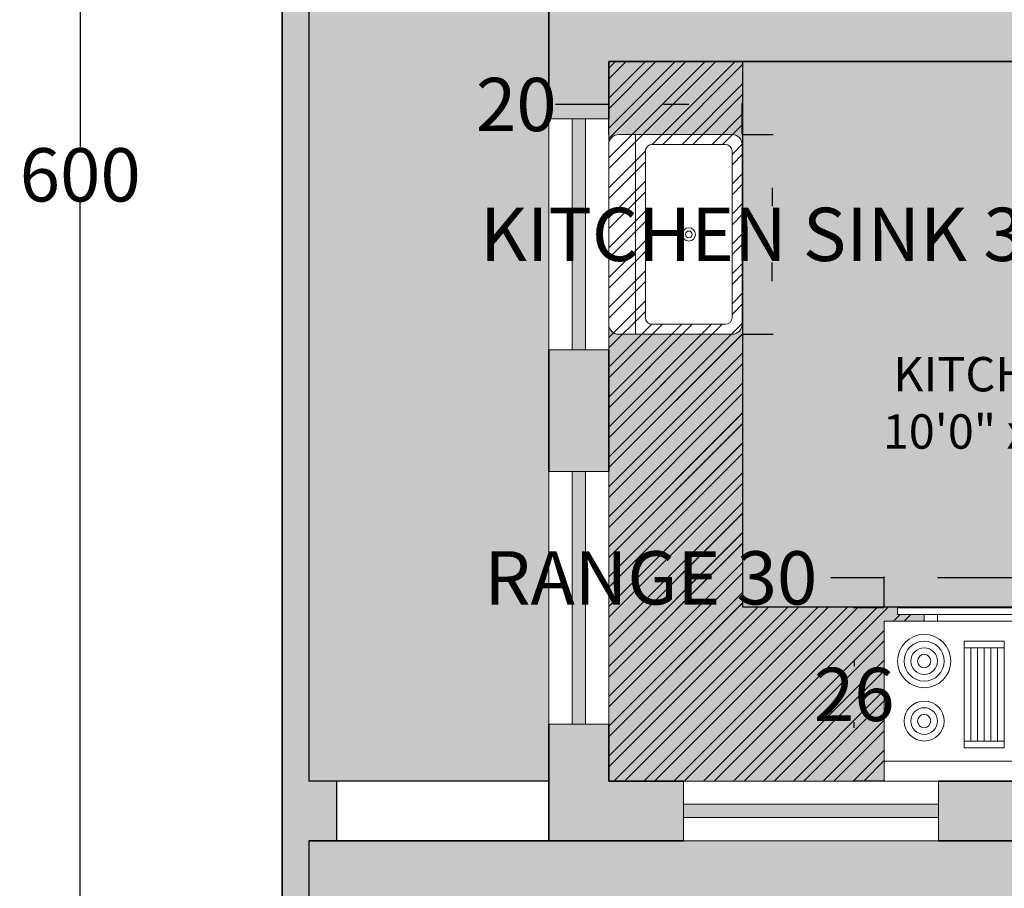
# Model space of a CAD drawing. Units: inches. Extents: x 389 to 971, y 148 to 870.
# Tile 7 of 14: x 389 to 537, y 428 to 558. Entities that reach past the tile are written whole.
import ezdxf

# ---------------------------------------------------------------- set-up
doc = ezdxf.new("R2010")
doc.units = ezdxf.units.IN
doc.header["$MEASUREMENT"] = 0
for name, color, linetype, lineweight in [('A-ANNO-DIMS', 2, 'Continuous', 18), ('A-AREA-IDEN', 7, 'Continuous', 18), ('A-CSWK-PATT', 9, 'Continuous', 13), ('A-EQPM', 8, 'Continuous', 18), ('A-FLOR-BASE-PATT', 8, 'Continuous', 13), ('A-FLOR-CSWK', 7, 'Continuous', 25), ('A-FLOR-FIXT', 8, 'Continuous', 18), ('A-GLAZ', 4, 'Continuous', 18), ('A-WALL', 7, 'Continuous', 35), ('C-PROP', 7, 'Continuous', 35), ('L-GRND-BASE-PATT', 8, 'Continuous', 13), ('L-WALL', 7, 'Continuous', 30)]:
    doc.layers.add(name, color=color, linetype=linetype, lineweight=lineweight)
for name, color, linetype, lineweight, true_color in [('A-CSWK-BASE-PATT', 18, 'Continuous', 13, 0x000000), ('A-GLAZ-PATT', 251, 'Continuous', 13, 0x6d5f6c), ('A-WALL-PATT', 18, 'Continuous', 13, 0x000000), ('L-GRND-PATT', 39, 'Continuous', 13, 0x603913)]:
    doc.layers.add(name, color=color, linetype=linetype, lineweight=lineweight, true_color=true_color)
doc.styles.get("Standard").update_dxf_attribs({"font": 'arial.ttf'})
doc.dimstyles.get("Standard").update_dxf_attribs({"dimtxt": 8, "dimasz": 8, "dimexe": 0.18, "dimexo": 0.0625, "dimgap": 0.09, "dimtad": 0, "dimtih": 1, "dimtoh": 1, "dimdec": 0, "dimzin": 0, "dimdsep": 46, "dimlunit": 3, "dimtxsty": 'Standard', "dimcen": 0.09, "dimadec": 0, "dimazin": 0, "dimtfac": 1, "dimtdec": 0, "dimtofl": 0, "dimtmove": 0, "dimatfit": 3, "dimfxl": 1, "dimtolj": 1, "dimtzin": 0, "dimarcsym": 0})
pattern_1 = [(45, (0, 0), (-2.245064, 2.245064), []), (45, (0, 1.5875), (-2.245064, 2.245064), [])]
pattern_2 = [(45, (0, 0), (0, 8.980256), [6.35, -6.35]), (45, (-1.684, 1.684), (0, 8.980256), [6.35, -6.35]), (45, (-3.3676, 3.3676), (0, 8.980256), [6.35, -6.35]), (135, (-3.3676, 4.49), (-8.980256, 0), [6.35, -6.35]), (135, (-1.684, 6.174), (-8.980256, 0), [6.35, -6.35]), (135, (0, 7.858), (-8.980256, 0), [6.35, -6.35])]

# ---------------------------------------------------------------- blocks, each defined once
blk = doc.blocks.new('Range-Oven - 30 in top')
for p, q in [((0, -3), (30, -3)), ((12, -6), (18, -6)), ((13, -20), (13, -6)), ((14, -6), (14, -20)), ((15, -20), (15, -6)), ((16, -6), (16, -20)), ((17, -20), (17, -6)), ((18, -20), (12, -20)), ((6, -24), (6, -25)), ((8, -25), (8, -24)), ((22, -25), (22, -24)), ((24, -24), (24, -25))]:
    blk.add_line(p, q)
for points in [[(0, -24), (0, 0), (30, 0), (30, -24)], [(12, -21), (12, -5), (18, -5), (18, -21)], [(2, -26), (2, -25), (28, -25), (28, -26)]]:
    blk.add_lwpolyline(points, close=True)
for centre, radius in [((6, -9), 4), ((6, -9), 3), ((6, -9), 2), ((24, -9), 3), ((24, -9), 2), ((6, -9), 1), ((24, -9), 1), ((24, -18), 4), ((6, -18), 3), ((6, -18), 2), ((24, -18), 3), ((24, -18), 2), ((6, -18), 1), ((24, -18), 1)]:
    blk.add_circle(centre, radius)
blk = doc.blocks.new('Sink-single - 30 in top')
blk.add_line((-15, -3.999996), (15, -3.999996))
for points in [[(-13.5, 0), (13.5, 0)], [(-15, -18.499996), (-15, -1.5)], [(15, -1.5), (15, -18.499996)], [(-12.5, -5.499996), (12.5, -5.499996)], [(-13.5, -17.499996), (-13.5, -6.499996)], [(13.5, -6.499996), (13.5, -17.499996)], [(12.5, -18.499996), (-12.5, -18.499996)], [(13.5, -19.999996), (-13.5, -19.999996)]]:
    blk.add_lwpolyline(points)
for radius in [1, 0.5]:
    blk.add_circle((0, -11.999996), radius)
for centre, radius, start, end in [((-13.5, -1.5), 1.5, 90, 180), ((13.5, -1.5), 1.5, 0, 90), ((-12.5, -6.499996), 1, 90, 180), ((12.5, -6.499996), 1, 0, 90), ((-12.5, -17.499996), 1, 180, 270), ((12.5, -17.499996), 1, 270, 0), ((-13.5, -18.499996), 1.5, 180, 270), ((13.5, -18.499996), 1.5, 270, 0)]:
    blk.add_arc(centre, radius, start, end)
blk = doc.blocks.new('*D32')
at = {"layer": 'A-ANNO-DIMS', "color": 0, "lineweight": -2, "transparency": 16777216}
for p, q in [((518.55, 474.14), (510.55, 474.14)), ((518.55, 469.71), (518.55, 474.32)), ((540.55, 474.14), (526.55, 474.14)), ((548.55, 469.71), (548.55, 474.32))]:
    blk.add_line(p, q, dxfattribs=at)
at = {"layer": 'A-ANNO-DIMS', "color": 0, "transparency": 16777216}
for points in [[(526.55, 475.48), (526.55, 472.81), (518.55, 474.14)], [(540.55, 475.48), (540.55, 472.81), (548.55, 474.14)]]:
    blk.add_solid(points, dxfattribs=at)
at = {"layer": 'Defpoints', "color": 0, "transparency": 16777216}
for p in [(518.55, 474.14), (518.55, 469.64), (548.55, 469.64)]:
    blk.add_point(p, dxfattribs=at)
at = {"layer": 'A-ANNO-DIMS', "color": 0, "transparency": 16777216, "insert": (483.53, 474.14), "char_height": 8, "attachment_point": 5}
blk.add_mtext('\\A1;RANGE 30', dxfattribs=at)
blk = doc.blocks.new('*D33')
at = {"layer": 'A-ANNO-DIMS', "color": 0, "lineweight": -2, "transparency": 16777216}
for p, q in [((518.49, 469.64), (513.87, 469.64)), ((514.05, 461.64), (514.05, 460.82)), ((514.05, 451.64), (514.05, 452.47)), ((518.49, 443.64), (513.87, 443.64))]:
    blk.add_line(p, q, dxfattribs=at)
at = {"layer": 'A-ANNO-DIMS', "color": 0, "transparency": 16777216}
for points in [[(512.72, 461.64), (515.39, 461.64), (514.05, 469.64)], [(512.72, 451.64), (515.39, 451.64), (514.05, 443.64)]]:
    blk.add_solid(points, dxfattribs=at)
at = {"layer": 'Defpoints', "color": 0, "transparency": 16777216}
for p in [(518.55, 469.64), (514.05, 443.64), (518.55, 443.64)]:
    blk.add_point(p, dxfattribs=at)
at = {"layer": 'A-ANNO-DIMS', "color": 0, "transparency": 16777216, "insert": (514.05, 456.64), "char_height": 8, "attachment_point": 5}
blk.add_mtext('\\A1;26', dxfattribs=at)
blk = doc.blocks.new('*D34')
at = {"layer": 'A-ANNO-DIMS', "color": 0, "lineweight": -2, "transparency": 16777216}
for p, q in [((497.28, 540.7), (501.9, 540.7)), ((501.72, 532.7), (501.72, 529.93)), ((501.72, 518.7), (501.72, 521.47)), ((497.28, 510.7), (501.9, 510.7))]:
    blk.add_line(p, q, dxfattribs=at)
at = {"layer": 'A-ANNO-DIMS', "color": 0, "transparency": 16777216}
for points in [[(500.38, 532.7), (503.05, 532.7), (501.72, 540.7)], [(500.38, 518.7), (503.05, 518.7), (501.72, 510.7)]]:
    blk.add_solid(points, dxfattribs=at)
at = {"layer": 'Defpoints', "color": 0, "transparency": 16777216}
for p in [(497.22, 540.7), (501.72, 540.7), (497.22, 510.7)]:
    blk.add_point(p, dxfattribs=at)
at = {"layer": 'A-ANNO-DIMS', "color": 0, "transparency": 16777216, "insert": (501.72, 525.7), "char_height": 8, "attachment_point": 5}
blk.add_mtext('\\A1;KITCHEN SINK 30', dxfattribs=at)
blk = doc.blocks.new('*D35')
at = {"layer": 'A-ANNO-DIMS', "color": 0, "lineweight": -2, "transparency": 16777216}
for p, q in [((477.22, 540.76), (477.22, 545.38)), ((497.22, 540.76), (497.22, 545.38)), ((477.22, 545.2), (469.22, 545.2)), ((489.22, 545.2), (485.22, 545.2))]:
    blk.add_line(p, q, dxfattribs=at)
at = {"layer": 'A-ANNO-DIMS', "color": 0, "transparency": 16777216}
for points in [[(485.22, 546.53), (485.22, 543.86), (477.22, 545.2)], [(489.22, 546.53), (489.22, 543.86), (497.22, 545.2)]]:
    blk.add_solid(points, dxfattribs=at)
at = {"layer": 'Defpoints', "color": 0, "transparency": 16777216}
for p in [(477.22, 545.2), (477.22, 540.7), (497.22, 540.7)]:
    blk.add_point(p, dxfattribs=at)
at = {"layer": 'A-ANNO-DIMS', "color": 0, "transparency": 16777216, "insert": (463.34, 545.2), "char_height": 8, "attachment_point": 5}
blk.add_mtext('\\A1;20', dxfattribs=at)
blk = doc.blocks.new('*D45')
at = {"layer": 'A-ANNO-DIMS', "color": 0, "lineweight": -2, "transparency": 16777216}
for p, q in [((428.15, 834.64), (397.71, 834.64)), ((397.89, 826.64), (397.89, 538.82)), ((397.89, 242.64), (397.89, 530.47)), ((428.15, 234.64), (397.71, 234.64))]:
    blk.add_line(p, q, dxfattribs=at)
at = {"layer": 'A-ANNO-DIMS', "color": 0, "transparency": 16777216}
for points in [[(396.56, 826.64), (399.22, 826.64), (397.89, 834.64)], [(396.56, 242.64), (399.22, 242.64), (397.89, 234.64)]]:
    blk.add_solid(points, dxfattribs=at)
at = {"layer": 'Defpoints', "color": 0, "transparency": 16777216}
for p in [(397.89, 834.64), (428.22, 834.64), (428.22, 234.64)]:
    blk.add_point(p, dxfattribs=at)
at = {"layer": 'A-ANNO-DIMS', "color": 0, "transparency": 16777216, "insert": (397.89, 534.64), "char_height": 8, "attachment_point": 5}
blk.add_mtext('\\A1;600', dxfattribs=at)

msp = doc.modelspace()

# ---------------------------------------------------------------- hatches: boundary and pattern name
at = {"layer": 'A-CSWK-BASE-PATT'}
h = msp.add_hatch(color=256, dxfattribs=at)
h.dxf.hatch_style = 1
h.paths.add_polyline_path([(477.216, 551.6445), (477.216, 543.0462), (477.216, 539.1979, -0.41421356), (478.716, 540.6979), (495.716, 540.6979, -0.41421356), (497.216, 539.1979), (497.3577, 551.6445)])
h = msp.add_hatch(color=256, dxfattribs=at)
h.dxf.hatch_style = 1
h.paths.add_polyline_path([(497.3577, 469.7503), (497.216, 512.1979, -0.41421356), (495.716, 510.6979), (478.716, 510.6979, -0.41421356), (477.216, 512.1979), (477.216, 508.3496), (477.216, 490.1255), (477.216, 452.1978), (477.216, 443.6445), (488.4095, 443.6445), (518.5523, 443.6445), (518.5523, 467.6445), (524.5523, 467.6445), (524.5523, 468.6445), (520.5523, 468.6445), (520.5523, 469.7503)])
at = {"layer": 'A-CSWK-PATT'}
h = msp.add_hatch(dxfattribs=at)
h.set_pattern_fill('STEEL', color=256)
h.set_pattern_definition(pattern_1)
h.paths.add_polyline_path([(477.216, 551.6445), (477.216, 543.0462), (477.216, 508.3496), (477.216, 490.1255), (477.216, 452.1978), (477.216, 443.6445), (488.4095, 443.6445), (526.7125, 443.6445), (540.3922, 443.6445), (585.0791, 443.6445), (595.387, 443.6445), (595.387, 515.7271), (574.1873, 515.7271), (574.1873, 469.7503), (497.3577, 469.7503), (497.3577, 551.6445)])
h.paths.add_polyline_path([(495.716, 540.6979, -0.41421356), (497.216, 539.1979), (497.216, 512.1979, -0.41421356), (495.716, 510.6979), (478.716, 510.6979, -0.41421356), (477.216, 512.1979), (477.216, 539.1979, -0.41421356), (478.716, 540.6979)], flags=0)
h.paths.add_polyline_path([(494.716, 539.1979, -0.41421356), (495.716, 538.1979), (495.716, 513.1979, -0.41421356), (494.716, 512.1979), (483.716, 512.1979, -0.41421356), (482.716, 513.1979), (482.716, 538.1979, -0.41421356), (483.716, 539.1979)], flags=16)
h.paths.add_polyline_path([(490.216, 525.6979, -1), (488.216, 525.6979, -1)], flags=0)
h.paths.add_polyline_path([(489.716, 525.6979, -1), (488.716, 525.6979, -1)], flags=0)
h.paths.add_polyline_path([(520.5523, 469.6445), (546.5523, 469.6445), (546.5523, 468.6445), (542.5523, 468.6445), (542.5523, 467.6445), (548.5523, 467.6445), (548.5523, 443.6445), (518.5523, 443.6445), (518.5523, 467.6445), (524.5523, 467.6445), (524.5523, 468.6445), (520.5523, 468.6445)], flags=16)
h.paths.add_polyline_path([(528.5523, 461.6445, -1), (520.5523, 461.6445, -1)], flags=0)
h.paths.add_polyline_path([(527.5523, 461.6445, -1), (521.5523, 461.6445, -1)], flags=0)
h.paths.add_polyline_path([(526.5523, 461.6445, -1), (522.5523, 461.6445, -1)], flags=0)
h.paths.add_polyline_path([(525.5523, 461.6445, -1), (523.5523, 461.6445, -1)], flags=0)
h.paths.add_polyline_path([(530.5523, 464.6445), (536.5523, 464.6445), (536.5523, 448.6445), (530.5523, 448.6445)], flags=0)
h.paths.add_polyline_path([(535.5523, 463.6445), (535.5523, 449.6445), (531.5523, 449.6445), (531.5523, 463.6445)], flags=0)
h.paths.add_polyline_path([(527.5523, 452.6445, -1), (521.5523, 452.6445, -1)], flags=0)
h.paths.add_polyline_path([(545.5523, 461.6445, -1), (539.5523, 461.6445, -1)], flags=0)
h.paths.add_polyline_path([(526.5523, 452.6445, -1), (522.5523, 452.6445, -1)], flags=0)
h.paths.add_polyline_path([(544.5523, 461.6445, -1), (540.5523, 461.6445, -1)], flags=0)
h.paths.add_polyline_path([(525.5523, 452.6445, -1), (523.5523, 452.6445, -1)], flags=0)
h.paths.add_polyline_path([(543.5523, 461.6445, -1), (541.5523, 461.6445, -1)], flags=0)
h.paths.add_polyline_path([(546.5523, 452.6445, -1), (538.5523, 452.6445, -1)], flags=0)
h.paths.add_polyline_path([(545.5523, 452.6445, -1), (539.5523, 452.6445, -1)], flags=0)
h.paths.add_polyline_path([(544.5523, 452.6445, -1), (540.5523, 452.6445, -1)], flags=0)
h.paths.add_polyline_path([(543.5523, 452.6445, -1), (541.5523, 452.6445, -1)], flags=0)
h = msp.add_hatch(dxfattribs=at)
h.set_pattern_fill('STEEL', color=256)
h.set_pattern_definition(pattern_1)
h.paths.add_polyline_path([(497.3577, 469.7503), (497.216, 512.1979, -0.41421356), (495.716, 510.6979), (478.716, 510.6979, -0.41421356), (477.216, 512.1979), (477.216, 508.3496), (477.216, 490.1255), (477.216, 452.1978), (477.216, 443.6445), (488.4095, 443.6445), (518.5523, 443.6445), (518.5523, 467.6445), (524.5523, 467.6445), (524.5523, 468.6445), (520.5523, 468.6445), (520.5523, 469.7503)])
at = {"layer": 'A-FLOR-BASE-PATT'}
h = msp.add_hatch(color=256, dxfattribs=at)
h.dxf.hatch_style = 1
h.paths.add_polyline_path([(497.3577, 469.7503), (574.1873, 469.7503), (574.1873, 515.7271), (595.387, 515.7271), (595.5252, 515.7478, -0.40276815), (565.4338, 544.4199), (565.4051, 544.4199), (565.4051, 545.7317), (595.387, 545.7317), (595.387, 551.6445), (497.3577, 551.6445)])
h.paths.add_polyline_path([(516.2555, 490.6064), (554.3542, 490.6064), (554.3542, 509.8575), (516.2555, 509.8575)], flags=24)
at = {"layer": 'A-GLAZ-PATT'}
h = msp.add_hatch(color=256, dxfattribs=at)
h.dxf.hatch_style = 1
h.paths.add_polyline_path([(473.716, 543.0462), (471.716, 543.0462), (471.716, 508.3496), (473.716, 508.3496)])
h = msp.add_hatch(color=256, dxfattribs=at)
h.dxf.hatch_style = 1
h.paths.add_polyline_path([(473.716, 490.1255), (471.716, 490.1255), (471.716, 452.1978), (473.716, 452.1978)])
h = msp.add_hatch(color=256, dxfattribs=at)
h.dxf.hatch_style = 1
h.paths.add_polyline_path([(488.4095, 440.1445), (488.4095, 438.1445), (526.7125, 438.1445), (526.7125, 440.1445)])
at = {"layer": 'A-WALL-PATT'}
h = msp.add_hatch(color=256, dxfattribs=at)
h.dxf.hatch_style = 1
h.paths.add_polyline_path([(432.216, 434.6445), (436.3673, 434.6445), (436.3673, 443.6445), (432.216, 443.6445), (432.216, 830.6445), (746.216, 830.6445), (746.216, 823.8175), (755.216, 823.8175), (755.216, 825.6445), (839.216, 825.6445), (839.216, 803.5176), (839.216, 741.6445), (755.216, 741.6445), (755.216, 748.4596), (755.1859, 748.4596), (750.716, 748.4596), (746.216, 748.4596), (746.216, 732.6445), (839.216, 732.6445), (839.216, 600.6445), (708.5171, 600.6445), (708.5171, 596.1445), (708.5171, 591.6445), (794.216, 591.6445), (794.216, 587.4291), (803.216, 587.4291), (803.216, 591.6445), (839.216, 591.6445), (839.216, 466.6012), (803.216, 466.6012), (803.216, 471.0309), (794.216, 471.0309), (794.216, 466.6012), (784.6145, 466.6012), (784.6145, 457.6012), (839.216, 457.6012), (839.216, 447.6445), (839.216, 294.6445), (810.0514, 294.6445), (810.0514, 285.6445), (839.216, 285.6445), (839.216, 238.6445), (590.216, 238.6445), (590.216, 234.6445), (848.216, 234.6445), (848.216, 834.6445), (428.216, 834.6445), (428.216, 234.6445), (437.216, 234.6445), (437.216, 243.6445), (432.216, 243.6445)])
h = msp.add_hatch(color=256, dxfattribs=at)
h.dxf.hatch_style = 1
h.paths.add_polyline_path([(538.3237, 641.6445), (538.3237, 637.1445), (538.3237, 632.6445), (595.387, 632.6445), (595.387, 560.6445), (558.5088, 560.6445), (511.387, 560.6445), (511.387, 585.4344), (502.387, 585.4344), (502.387, 560.6445), (468.216, 560.6445), (468.216, 543.0462), (477.216, 543.0462), (477.216, 551.6445), (595.387, 551.6445), (595.387, 545.7317), (595.3894, 545.7317), (599.887, 545.7317), (604.387, 545.7317), (604.387, 632.6445), (619.5147, 632.6445), (619.5147, 641.6445)])
h = msp.add_hatch(color=256, dxfattribs=at)
h.dxf.hatch_style = 1
h.paths.add_polyline_path([(477.216, 508.3496), (468.216, 508.3496), (468.216, 490.1255), (477.216, 490.1255)])
h = msp.add_hatch(color=256, dxfattribs=at)
h.dxf.hatch_style = 1
h.paths.add_polyline_path([(477.216, 443.6445), (477.216, 452.1978), (468.216, 452.1978), (468.216, 434.6445), (488.4095, 434.6445), (488.4095, 443.6445)])
h = msp.add_hatch(color=256, dxfattribs=at)
h.dxf.hatch_style = 1
h.paths.add_polyline_path([(540.3922, 434.6445), (540.3922, 443.6445), (526.7125, 443.6445), (526.7125, 434.6445)])
at = {"layer": 'L-GRND-BASE-PATT'}
h = msp.add_hatch(color=256, dxfattribs=at)
h.dxf.hatch_style = 1
h.paths.add_polyline_path([(468.216, 560.6445), (502.387, 560.6445), (502.387, 585.4344), (502.387, 613.354), (502.387, 632.6445), (468.216, 632.6445), (468.216, 651.2738), (468.216, 699.1491), (468.216, 728.9805), (468.216, 777.4428), (468.216, 794.6445), (534.7176, 794.6445), (606.2724, 794.6445), (685.2392, 794.6445), (734.7772, 794.6445), (746.216, 794.6445), (746.216, 796.191), (746.216, 823.8175), (746.216, 830.6445), (432.216, 830.6445), (432.216, 443.6445), (468.216, 443.6445), (468.216, 452.1978), (468.216, 490.1255), (468.216, 508.3496), (468.216, 543.0462)])
h.paths.add_polyline_path([(456.8918, 600.1849), (456.8918, 677.4216), (446.55, 677.4216), (446.55, 600.1849)], flags=24)
h.paths.add_polyline_path([(573.4326, 807.2886), (651.063, 807.2886), (651.063, 817.6304), (573.4326, 817.6304)], flags=24)
h = msp.add_hatch(color=256, dxfattribs=at)
h.dxf.hatch_style = 1
edge = h.paths.add_edge_path(flags=16)
edge.add_ellipse((8782.0026, 354.2473), major_axis=(-8296.9493, 0), ratio=0.84230387, start_angle=-0.09022909, end_angle=0.38386678, ccw=False)
edge.add_ellipse((485.0533, 368.2895), major_axis=(-1.1591, 0), ratio=0.84230387, start_angle=0, end_angle=90, ccw=False)
edge.add_line((483.8943, 368.2895), (483.8943, 387.6039))
edge.add_ellipse((485.0533, 387.2466), major_axis=(1.1591, 0), ratio=0.84230387, start_angle=90, end_angle=180, ccw=False)
edge.add_line((485.0533, 388.2229), (485.5047, 388.2229))
edge.add_ellipse((898.8202, 372.4897), major_axis=(413.7374, 0), ratio=0.84230387, start_angle=176.349572, end_angle=177.82005, ccw=False)
edge.add_ellipse((535.9119, 196.3855), major_axis=(-245.3972, 0), ratio=0.84230387, start_angle=-77.874034, end_angle=-76.219471, ccw=False)
edge.add_ellipse((535.9119, 201.7547), major_axis=(239.1274, 0), ratio=0.84230387, start_angle=100.209539, end_angle=102.444627, ccw=False)
edge.add_ellipse((473.3139, 564.9222), major_axis=(196.5637, 0), ratio=0.84230387, start_angle=-80.743434, end_angle=-77.445067)
edge.add_line((509.5535, 402.1941), (514.3535, 404.8483))
edge.add_line((514.3535, 404.8483), (514.3535, 404.7972))
edge.add_ellipse((514.3535, 404.2644), major_axis=(0.5795, 0), ratio=0.84230387, start_angle=52.06687, end_angle=90, ccw=False)
edge.add_line((514.6716, 404.6725), (519.1535, 402.1941))
edge.add_ellipse((555.3932, 564.9222), major_axis=(-196.5637, 0), ratio=0.84230387, start_angle=77.445067, end_angle=80.743434)
edge.add_ellipse((492.7951, 201.7547), major_axis=(239.1274, 0), ratio=0.84230387, start_angle=77.555373, end_angle=79.790461, ccw=False)
edge.add_ellipse((492.7951, 196.3855), major_axis=(245.3972, 0), ratio=0.84230387, start_angle=76.219471, end_angle=77.874034, ccw=False)
edge.add_ellipse((129.8868, 372.4897), major_axis=(-413.7374, 0), ratio=0.84230387, start_angle=182.17995, end_angle=183.650428, ccw=False)
edge.add_line((543.2023, 388.2229), (544.0779, 388.2229))
edge.add_ellipse((543.6537, 387.2466), major_axis=(-1.1591, 0), ratio=0.84230387, start_angle=180, end_angle=270, ccw=False)
edge.add_line((544.8128, 387.2466), (544.8128, 367.9322))
edge.add_ellipse((543.6537, 368.2895), major_axis=(1.1591, 0), ratio=0.84230387, start_angle=270, end_angle=360, ccw=False)
edge.add_ellipse((-7753.2956, 354.2473), major_axis=(-8296.9493, 0), ratio=0.84230387, start_angle=179.61613322, end_angle=180.09022909, ccw=False)
edge.add_line((543.3912, 298.6608), (544.0779, 298.6608))
edge.add_ellipse((543.6537, 297.6845), major_axis=(1.1591, 0), ratio=0.84230387, start_angle=0, end_angle=90, ccw=False)
edge.add_line((544.8128, 297.6845), (544.8128, 278.3701))
edge.add_ellipse((543.6537, 278.7275), major_axis=(-1.1591, 0), ratio=0.84230387, start_angle=90, end_angle=180, ccw=False)
edge.add_line((543.6537, 277.7512), (543.1566, 277.7512))
edge.add_ellipse((-7753.2956, 354.2473), major_axis=(-8296.9493, 0), ratio=0.84230387, start_angle=179.3813568, end_angle=179.47172853, ccw=False)
edge.add_ellipse((542.4236, 263.2763), major_axis=(-1.7386, 0), ratio=0.84230387, start_angle=179.371763, end_angle=248.464757, ccw=False)
edge.add_ellipse((-7753.8751, 354.2473), major_axis=(-8298.7403, 0), ratio=0.842303866, start_angle=179.35344592, end_angle=179.3717628, ccw=False)
edge.add_ellipse((540.0116, 260.6509), major_axis=(-4.1092, 0), ratio=0.84230387, start_angle=90, end_angle=179.353446, ccw=False)
edge.add_line((540.0116, 257.1897), (488.6954, 257.1897))
edge.add_ellipse((488.6954, 260.6509), major_axis=(4.1092, 0), ratio=0.84230387, start_angle=180.646554, end_angle=270, ccw=False)
edge.add_ellipse((8782.5821, 354.2473), major_axis=(-8298.7403, 0), ratio=0.842303872, start_angle=0.62823723, end_angle=0.64655411, ccw=False)
edge.add_ellipse((486.2834, 263.2763), major_axis=(-1.7386, 0), ratio=0.84230387, start_angle=-68.464756, end_angle=0.628237, ccw=False)
edge.add_ellipse((8782.0026, 354.2473), major_axis=(-8296.9493, 0), ratio=0.84230387, start_angle=0.52827147, end_angle=0.6465541, ccw=False)
edge.add_line((485.5504, 277.7512), (484.6291, 277.7512))
edge.add_ellipse((485.0533, 278.7275), major_axis=(-1.1591, 0), ratio=0.84230387, start_angle=0, end_angle=90, ccw=False)
edge.add_line((483.8943, 278.7275), (483.8943, 298.0418))
edge.add_ellipse((485.0533, 297.6845), major_axis=(1.1591, 0), ratio=0.84230387, start_angle=90, end_angle=180, ccw=False)
edge = h.paths.add_edge_path(flags=0)
edge.add_ellipse((8782.0026, 354.2473), major_axis=(-8295.7902, 0), ratio=0.84230387, start_angle=0.05559431, end_angle=0.37776419, ccw=False)
edge.add_line((486.2179, 346.1978), (489.3905, 335.8384))
edge.add_ellipse((3386.0114, 329.7263), major_axis=(-2896.63, 0), ratio=0.84230387, start_angle=-0.1208974, end_angle=0.3640763)
edge.add_line((489.4638, 311.3204), (486.4666, 299.5521))
edge = h.paths.add_edge_path(flags=0)
edge.add_ellipse((514.3535, 391.3731), major_axis=(-115.1513, 0), ratio=0.84230387, start_angle=76.401865, end_angle=103.598135)
edge.add_line((537.3428, 296.3333), (537.3428, 281.5897))
edge.add_ellipse((514.3535, 376.6295), major_axis=(-115.1513, 0), ratio=0.84230387, start_angle=76.401865, end_angle=103.598135, ccw=False)
edge.add_line((491.3643, 281.5897), (491.3643, 296.3333))
edge = h.paths.add_edge_path(flags=0)
edge.add_line((491.3643, 337.0752), (489.653, 349.9016))
edge.add_ellipse((510.1338, 298.7862), major_axis=(64.0481, 0), ratio=0.84230387, start_angle=94.277421, end_angle=111.834954, ccw=False)
edge.add_line((506.1068, 352.6274), (522.6002, 352.6274))
edge.add_ellipse((518.5732, 298.7862), major_axis=(64.0481, 0), ratio=0.84230387, start_angle=68.165046, end_angle=85.722579, ccw=False)
edge.add_line((539.0541, 349.9016), (537.3428, 337.0752))
edge.add_ellipse((516.5462, 287.5825), major_axis=(62.3305, 0), ratio=0.84230387, start_angle=67.208085, end_angle=85.12993)
edge.add_line((521.008, 339.949), (507.699, 339.949))
edge.add_ellipse((512.1609, 287.5825), major_axis=(62.3305, 0), ratio=0.84230387, start_angle=94.87007, end_angle=112.791915)
edge = h.paths.add_edge_path(flags=0)
edge.add_ellipse((493.6824, 273.9439), major_axis=(-2.3182, 0), ratio=0.84230387, start_angle=-90, end_angle=0, ccw=False)
edge.add_line((493.6824, 275.8965), (535.3743, 275.8965))
edge.add_ellipse((535.0246, 273.9439), major_axis=(2.3182, 0), ratio=0.84230387, start_angle=0, end_angle=90, ccw=False)
edge.add_line((537.3428, 273.9439), (537.3428, 258.6983))
edge.add_line((537.3428, 258.6983), (540.5912, 258.6983))
edge.add_ellipse((540.5912, 260.6509), major_axis=(-2.3182, 0), ratio=0.84230387, start_angle=90, end_angle=179.353446)
edge.add_line((540.5912, 258.6983), (487.7691, 258.6983))
edge.add_ellipse((488.1158, 260.6509), major_axis=(2.3182, 0), ratio=0.84230387, start_angle=180.646554, end_angle=270)
edge.add_line((488.1158, 258.6983), (491.3643, 258.6983))
edge.add_line((491.3643, 258.6983), (491.3643, 274.2384))
h.paths.add_polyline_path([(746.1376, 327.3223), (750.14, 327.3223), (750.14, 326.2831), (798.1694, 326.2831), (798.1694, 327.3223), (802.1718, 327.3223), (802.1718, 309.9784, -0.19047621), (746.1376, 309.9784)], flags=16)
h.paths.add_polyline_path([(782.1596, 313.5685), (782.1596, 309.0415, -0.04962821), (766.1498, 309.0415), (766.1498, 313.5685)], flags=0)
h.paths.add_polyline_path([(755.1859, 344.9352), (755.1859, 373.9163), (788.1244, 373.9163), (788.1244, 344.9352)], flags=16)
h.paths.add_polyline_path([(757.1859, 346.9352), (757.1859, 371.9163), (786.1244, 371.9163), (786.1244, 346.9352)], flags=0)
h.paths.add_polyline_path([(803.6446, 338.4879), (803.6446, 342.4903), (804.6838, 342.4903), (804.6838, 390.5197), (803.6446, 390.5197), (803.6446, 394.5221), (820.9885, 394.5221, -0.19047621), (820.9885, 338.4879)], flags=16)
h.paths.add_polyline_path([(806.8707, 326.6963), (806.4254, 327.1416), (806.4724, 326.6297)], flags=16)
h.paths.add_polyline_path([(822.0328, 317.4008), (822.1942, 317.8933), (821.5626, 317.9885)], flags=16)
h.paths.add_polyline_path([(817.3984, 358.5001), (817.3984, 374.5099), (821.9254, 374.5099, -0.04962821), (821.9254, 358.5001)], flags=0)
h.paths.add_polyline_path([(808.1446, 418.9737), (808.2247, 418.5632), (808.5395, 418.5787)], flags=16)
h.paths.add_polyline_path([(820.3159, 412.669), (820.4772, 413.1615), (819.8457, 413.2568)], flags=16)
h.paths.add_polyline_path([(466.3155, 235.5246), (517.3807, 235.5246), (517.3807, 244.4269), (466.3155, 244.4269)], flags=24)
h.paths.add_polyline_path([(739.8737, 256.2), (815.404, 256.2), (815.404, 265.3454), (739.8737, 265.3454)], flags=24)
h.paths.add_polyline_path([(750.6082, 393.6667), (791.5681, 393.6667), (791.5681, 412.3933), (750.6082, 412.3933)], flags=24)
h.paths.add_polyline_path([(438.9631, 410.0619), (484.6204, 410.0619), (484.6204, 429.1217), (438.9631, 429.1217)], flags=24)
edge = h.paths.add_edge_path()
edge.add_line((839.216, 285.6445), (611.8787, 285.6445))
edge.add_line((611.8787, 285.6445), (604.387, 285.6445))
edge.add_line((604.387, 285.6445), (595.387, 285.6445))
edge.add_line((595.387, 285.6445), (595.387, 370.1554))
edge.add_line((595.387, 370.1554), (604.0817, 370.1554))
edge.add_line((604.0817, 370.1554), (604.0817, 371.3788))
edge.add_line((604.0817, 371.3788), (632.0195, 371.3788))
edge.add_arc((604.0817, 370.1554), 27.9645, 2.507491, 90)
edge.add_line((604.0817, 398.1199), (599.887, 398.1652))
edge.add_line((599.887, 398.1652), (604.4225, 398.1652))
edge.add_arc((604.4225, 428.4021), 30.2369, 270, 357.492509)
edge.add_line((634.6305, 427.0792), (604.4225, 427.0792))
edge.add_line((604.4225, 427.0792), (604.4225, 428.4021))
edge.add_line((604.4225, 428.4021), (599.887, 428.4021))
edge.add_line((599.887, 428.4021), (595.387, 428.4021))
edge.add_line((595.387, 428.4021), (595.387, 434.6445))
edge.add_line((595.387, 434.6445), (585.0791, 434.6445))
edge.add_line((585.0791, 434.6445), (540.3922, 434.6445))
edge.add_line((540.3922, 434.6445), (526.7125, 434.6445))
edge.add_line((526.7125, 434.6445), (488.4095, 434.6445))
edge.add_line((488.4095, 434.6445), (432.216, 434.6445))
edge.add_line((432.216, 434.6445), (432.216, 243.6445))
edge.add_line((432.216, 243.6445), (437.216, 243.6445))
edge.add_line((437.216, 243.6445), (437.216, 234.6445))
edge.add_line((437.216, 234.6445), (581.216, 234.6445))
edge.add_line((581.216, 234.6445), (581.216, 238.6445))
edge.add_line((581.216, 238.6445), (581.216, 243.6445))
edge.add_line((581.216, 243.6445), (590.216, 243.6445))
edge.add_line((590.216, 243.6445), (590.216, 238.6445))
edge.add_line((590.216, 238.6445), (839.216, 238.6445))
edge.add_line((839.216, 238.6445), (839.216, 285.6445))
at = {"layer": 'L-GRND-PATT'}
h = msp.add_hatch(dxfattribs=at)
h.set_pattern_fill('EARTH', color=256, angle=45)
h.set_pattern_definition(pattern_2)
h.paths.add_polyline_path([(468.216, 560.6445), (502.387, 560.6445), (502.387, 585.4344), (502.387, 613.354), (502.387, 632.6445), (468.216, 632.6445), (468.216, 651.2738), (468.216, 699.1491), (468.216, 728.9805), (468.216, 777.4428), (468.216, 794.6445), (534.7176, 794.6445), (606.2724, 794.6445), (685.2392, 794.6445), (734.7772, 794.6445), (746.216, 794.6445), (746.216, 796.191), (746.216, 823.8175), (746.216, 830.6445), (432.216, 830.6445), (432.216, 443.6445), (468.216, 443.6445), (468.216, 452.1978), (468.216, 490.1255), (468.216, 508.3496), (468.216, 543.0462)])
h.paths.add_polyline_path([(456.8918, 600.1849), (456.8918, 677.4216), (446.55, 677.4216), (446.55, 600.1849)], flags=24)
h.paths.add_polyline_path([(573.4326, 807.2886), (651.063, 807.2886), (651.063, 817.6304), (573.4326, 817.6304)], flags=24)
h = msp.add_hatch(dxfattribs=at)
h.set_pattern_fill('EARTH', color=256, angle=45)
h.set_pattern_definition(pattern_2)
h.paths.add_polyline_path([(432.216, 243.6445), (437.216, 243.6445), (437.216, 234.6445), (581.216, 234.6445), (581.216, 238.6445), (581.216, 243.6445), (590.216, 243.6445), (590.216, 238.6445), (839.216, 238.6445), (839.216, 285.6445), (810.0514, 285.6445), (733.8057, 285.6445), (684.2434, 285.6445), (611.8787, 285.6445), (604.387, 285.6445), (595.387, 285.6445), (595.387, 370.1554), (604.0817, 370.1554), (604.0817, 371.3788), (632.0195, 371.3788, 0.40145271), (604.0817, 398.1199), (599.887, 398.1652), (604.4225, 398.1652, 0.40145271), (634.6305, 427.0792), (604.4225, 427.0792), (604.4225, 428.4021), (599.887, 428.4021), (595.387, 428.4021), (595.387, 434.6445), (585.0791, 434.6445), (540.3922, 434.6445), (526.7125, 434.6445), (488.4095, 434.6445), (432.216, 434.6445)])
edge = h.paths.add_edge_path(flags=16)
edge.add_line((483.8943, 278.7275), (483.8943, 298.2564))
edge.add_ellipse((485.0533, 297.6845), major_axis=(1.1591, 0), ratio=0.84230387, start_angle=90, end_angle=180, ccw=False)
edge.add_ellipse((8782.0026, 354.2473), major_axis=(-8296.9493, 0), ratio=0.84230387, start_angle=-0.09022909, end_angle=0.38386678, ccw=False)
edge.add_ellipse((485.0533, 368.2895), major_axis=(-1.1591, 0), ratio=0.84230387, start_angle=0, end_angle=90, ccw=False)
edge.add_line((483.8943, 368.2895), (483.8943, 387.8185))
edge.add_ellipse((485.0533, 387.2466), major_axis=(1.1591, 0), ratio=0.84230387, start_angle=90, end_angle=180, ccw=False)
edge.add_ellipse((898.8202, 372.4897), major_axis=(413.7374, 0), ratio=0.84230387, start_angle=176.349572, end_angle=177.82005, ccw=False)
edge.add_ellipse((535.9119, 196.3855), major_axis=(-245.3972, 0), ratio=0.84230387, start_angle=-77.874034, end_angle=-76.219471, ccw=False)
edge.add_ellipse((535.9119, 201.7547), major_axis=(239.1274, 0), ratio=0.84230387, start_angle=100.209539, end_angle=102.444627, ccw=False)
edge.add_ellipse((473.3139, 564.9222), major_axis=(196.5637, 0), ratio=0.84230387, start_angle=-80.743434, end_angle=-77.445067)
edge.add_line((509.5535, 402.1941), (514.3535, 404.8483))
edge.add_line((514.3535, 404.8483), (519.1535, 402.1941))
edge.add_ellipse((555.3932, 564.9222), major_axis=(-196.5637, 0), ratio=0.84230387, start_angle=77.445067, end_angle=80.743434)
edge.add_ellipse((492.7951, 201.7547), major_axis=(239.1274, 0), ratio=0.84230387, start_angle=77.555373, end_angle=79.790461, ccw=False)
edge.add_ellipse((492.7951, 196.3855), major_axis=(245.3972, 0), ratio=0.84230387, start_angle=76.219471, end_angle=77.874034, ccw=False)
edge.add_ellipse((129.8868, 372.4897), major_axis=(-413.7374, 0), ratio=0.84230387, start_angle=182.17995, end_angle=183.650428, ccw=False)
edge.add_line((543.2023, 388.2229), (544.3327, 388.2229))
edge.add_ellipse((543.6537, 387.2466), major_axis=(-1.1591, 0), ratio=0.84230387, start_angle=180, end_angle=270, ccw=False)
edge.add_line((544.8128, 387.2466), (544.8128, 367.7176))
edge.add_ellipse((543.6537, 368.2895), major_axis=(1.1591, 0), ratio=0.84230387, start_angle=270, end_angle=360, ccw=False)
edge.add_ellipse((-7753.2956, 354.2473), major_axis=(-8296.9493, 0), ratio=0.84230387, start_angle=179.61613322, end_angle=180.09022909, ccw=False)
edge.add_ellipse((543.6537, 297.6845), major_axis=(1.1591, 0), ratio=0.84230387, start_angle=0, end_angle=90, ccw=False)
edge.add_line((544.8128, 297.6845), (544.8128, 278.1556))
edge.add_ellipse((543.6537, 278.7275), major_axis=(-1.1591, 0), ratio=0.84230387, start_angle=90, end_angle=180, ccw=False)
edge.add_ellipse((-7753.2956, 354.2473), major_axis=(-8296.9493, 0), ratio=0.84230387, start_angle=179.3813568, end_angle=179.47172853, ccw=False)
edge.add_ellipse((542.4236, 263.2763), major_axis=(-1.7386, 0), ratio=0.84230387, start_angle=179.371763, end_angle=248.464757, ccw=False)
edge.add_ellipse((-7753.8751, 354.2473), major_axis=(-8298.7403, 0), ratio=0.842303866, start_angle=179.35344592, end_angle=179.3717628, ccw=False)
edge.add_ellipse((540.0116, 260.6509), major_axis=(-4.1092, 0), ratio=0.84230387, start_angle=90, end_angle=179.353446, ccw=False)
edge.add_line((540.0116, 257.1897), (488.0808, 257.1897))
edge.add_ellipse((488.6954, 260.6509), major_axis=(4.1092, 0), ratio=0.84230387, start_angle=180.646554, end_angle=270, ccw=False)
edge.add_ellipse((8782.5821, 354.2473), major_axis=(-8298.7403, 0), ratio=0.842303872, start_angle=0.62823723, end_angle=0.64655411, ccw=False)
edge.add_ellipse((486.2834, 263.2763), major_axis=(-1.7386, 0), ratio=0.84230387, start_angle=-68.464756, end_angle=0.628237, ccw=False)
edge.add_ellipse((8782.0026, 354.2473), major_axis=(-8296.9493, 0), ratio=0.84230387, start_angle=0.52827147, end_angle=0.6465541, ccw=False)
edge.add_line((485.5504, 277.7512), (484.3744, 277.7512))
edge.add_ellipse((485.0533, 278.7275), major_axis=(-1.1591, 0), ratio=0.84230387, start_angle=0, end_angle=90, ccw=False)
edge = h.paths.add_edge_path(flags=0)
edge.add_ellipse((488.1158, 260.6509), major_axis=(2.3182, 0), ratio=0.84230387, start_angle=180.646554, end_angle=270)
edge.add_line((488.1158, 258.6983), (491.3643, 258.6983))
edge.add_line((491.3643, 258.6983), (491.3643, 274.4686))
edge.add_ellipse((493.6824, 273.9439), major_axis=(-2.3182, 0), ratio=0.84230387, start_angle=-90, end_angle=0, ccw=False)
edge.add_line((493.6824, 275.8965), (535.6476, 275.8965))
edge.add_ellipse((535.0246, 273.9439), major_axis=(2.3182, 0), ratio=0.84230387, start_angle=0, end_angle=90, ccw=False)
edge.add_line((537.3428, 273.9439), (537.3428, 258.6983))
edge.add_line((537.3428, 258.6983), (541.2086, 258.6983))
edge.add_ellipse((540.5912, 260.6509), major_axis=(-2.3182, 0), ratio=0.84230387, start_angle=90, end_angle=179.353446, ccw=False)
edge.add_line((540.5912, 258.6983), (487.4984, 258.6983))
edge = h.paths.add_edge_path(flags=0)
edge.add_line((491.3643, 281.5897), (491.3643, 296.3333))
edge.add_ellipse((514.3535, 391.3731), major_axis=(-115.1513, 0), ratio=0.84230387, start_angle=76.401865, end_angle=103.598135)
edge.add_line((537.3428, 296.3333), (537.3428, 281.5897))
edge.add_ellipse((514.3535, 376.6295), major_axis=(-115.1513, 0), ratio=0.84230387, start_angle=76.401865, end_angle=103.598135, ccw=False)
edge = h.paths.add_edge_path(flags=0)
edge.add_ellipse((8782.0026, 354.2473), major_axis=(-8295.7902, 0), ratio=0.84230387, start_angle=0.05559431, end_angle=0.37776419, ccw=False)
edge.add_line((486.2179, 346.1978), (489.3905, 335.8384))
edge.add_ellipse((3386.0114, 329.7263), major_axis=(-2896.63, 0), ratio=0.84230387, start_angle=-0.1208974, end_angle=0.3640763)
edge.add_line((489.4638, 311.3204), (486.4666, 299.5521))
edge = h.paths.add_edge_path(flags=0)
edge.add_line((491.3643, 337.0752), (489.653, 349.9016))
edge.add_ellipse((510.1338, 298.7862), major_axis=(64.0481, 0), ratio=0.84230387, start_angle=94.277421, end_angle=111.834954, ccw=False)
edge.add_line((506.1068, 352.6274), (522.6002, 352.6274))
edge.add_ellipse((518.5732, 298.7862), major_axis=(64.0481, 0), ratio=0.84230387, start_angle=68.165046, end_angle=85.722579, ccw=False)
edge.add_line((539.0541, 349.9016), (537.3428, 337.0752))
edge.add_ellipse((516.5462, 287.5825), major_axis=(62.3305, 0), ratio=0.84230387, start_angle=67.208085, end_angle=85.12993)
edge.add_line((521.008, 339.949), (507.699, 339.949))
edge.add_ellipse((512.1609, 287.5825), major_axis=(62.3305, 0), ratio=0.84230387, start_angle=94.87007, end_angle=112.791915)
h.paths.add_polyline_path([(466.3155, 235.5246), (517.3807, 235.5246), (517.3807, 244.4269), (466.3155, 244.4269)], flags=24)
h.paths.add_polyline_path([(739.8737, 256.2), (815.404, 256.2), (815.404, 265.3454), (739.8737, 265.3454)], flags=24)
h.paths.add_polyline_path([(438.9631, 410.0619), (484.6204, 410.0619), (484.6204, 429.1217), (438.9631, 429.1217)], flags=24)

# ---------------------------------------------------------------- linework, layer by layer
at = {"layer": 'A-FLOR-CSWK'}
for p, q in [((497.3577, 469.7503), (497.3577, 551.6445)), ((574.1873, 469.7503), (497.3577, 469.7503))]:
    msp.add_line(p, q, dxfattribs=at)
at = {"layer": 'A-GLAZ'}
for p, q in [((477.216, 543.0462), (468.216, 543.0462)), ((468.216, 543.0462), (468.216, 508.3496)), ((471.716, 543.0462), (471.716, 508.3496)), ((473.716, 543.0462), (473.716, 508.3496)), ((477.216, 543.0462), (477.216, 508.3496)), ((477.216, 508.3496), (468.216, 508.3496)), ((477.216, 490.1255), (468.216, 490.1255)), ((468.216, 490.1255), (468.216, 452.1978)), ((471.716, 490.1255), (471.716, 452.1978)), ((473.716, 490.1255), (473.716, 452.1978)), ((477.216, 490.1255), (477.216, 452.1978)), ((477.216, 452.1978), (468.216, 452.1978)), ((488.4095, 443.6445), (488.4095, 434.6445)), ((488.4095, 443.6445), (526.7125, 443.6445)), ((526.7125, 443.6445), (526.7125, 434.6445)), ((488.4095, 440.1445), (526.7125, 440.1445)), ((488.4095, 438.1445), (526.7125, 438.1445)), ((488.4095, 434.6445), (526.7125, 434.6445))]:
    msp.add_line(p, q, dxfattribs=at)
at = {"layer": 'A-WALL'}
for p, q in [((468.216, 560.6445), (468.216, 543.0462)), ((477.216, 551.6445), (477.216, 543.0462)), ((595.387, 551.6445), (477.216, 551.6445)), ((468.216, 508.3496), (468.216, 490.1255)), ((477.216, 508.3496), (477.216, 490.1255)), ((468.216, 452.1978), (468.216, 434.6445)), ((477.216, 452.1978), (477.216, 443.6445)), ((488.4095, 443.6445), (477.216, 443.6445)), ((540.3922, 443.6445), (526.7125, 443.6445)), ((488.4095, 434.6445), (432.216, 434.6445)), ((540.3922, 434.6445), (526.7125, 434.6445))]:
    msp.add_line(p, q, dxfattribs=at)
at = {"layer": 'C-PROP'}
msp.add_line((428.216, 834.6445), (428.216, 234.6445), dxfattribs=at)
at = {"layer": 'L-WALL'}
for p, q in [((432.216, 830.6445), (432.216, 443.6445)), ((468.216, 443.6445), (432.216, 443.6445)), ((436.3673, 443.6445), (436.3673, 434.6445)), ((432.216, 434.6445), (432.216, 294.6445))]:
    msp.add_line(p, q, dxfattribs=at)

# ---------------------------------------------------------------- block references
at = {"layer": 'A-EQPM', "rotation": 180}
msp.add_blockref('Range-Oven - 30 in top', (548.5523, 443.6445), dxfattribs=at)
at = {"layer": 'A-FLOR-FIXT', "rotation": 90}
msp.add_blockref('Sink-single - 30 in top', (477.216, 525.6979), dxfattribs=at)

# ---------------------------------------------------------------- texts
at = {"layer": 'A-AREA-IDEN', "insert": (518.33, 507.2902), "char_height": 5.159132, "attachment_point": 1}
msp.add_mtext_dynamic_manual_height_columns(' KITCHEN\\P10\'0" x 9\'0"', width=117.090289, gutter_width=25.7957, heights=[0], dxfattribs=at)

# ---------------------------------------------------------------- dimensions: what is measured, and where the dimension line sits
at = {"layer": 'A-ANNO-DIMS'}
for base, p1, p2, angle, picture, middle in [((397.891, 834.6445), (428.216, 234.6445), (428.216, 834.6445), 90, '*D45', (397.891, 534.6445)), ((477.216, 545.1979), (497.216, 540.6979), (477.216, 540.6979), 180, '*D35', (463.3416, 545.1979)), ((514.0523, 443.6445), (518.5523, 469.6445), (518.5523, 443.6445), 270, '*D33', (514.0523, 456.6445))]:
    dim = msp.add_linear_dim(base=base, p1=p1, p2=p2, angle=angle, dimstyle='Standard', override={"dimdec": 0, "dimlfac": 1, "dimrnd": 0, "dimzin": 0, "dimdsep": 46, "dimlunit": 2}, dxfattribs=at)
    dim.commit()
    dim.dimension.update_dxf_attribs({"geometry": picture, "text_midpoint": middle})
for base, p1, p2, angle, text, picture, middle in [((501.716, 540.6979), (497.216, 510.6979), (497.216, 540.6979), 90, 'KITCHEN SINK <>', '*D34', (501.716, 525.6979)), ((518.5523, 474.1445), (548.5523, 469.6445), (518.5523, 469.6445), 180, 'RANGE <>', '*D32', (483.5292, 474.1445))]:
    dim = msp.add_linear_dim(base=base, p1=p1, p2=p2, angle=angle, text=text, dimstyle='Standard', override={"dimdec": 0, "dimlfac": 1, "dimrnd": 0, "dimzin": 0, "dimdsep": 46, "dimlunit": 2}, dxfattribs=at)
    dim.commit()
    dim.dimension.update_dxf_attribs({"geometry": picture, "text_midpoint": middle})

doc.saveas('drawing.dxf')
